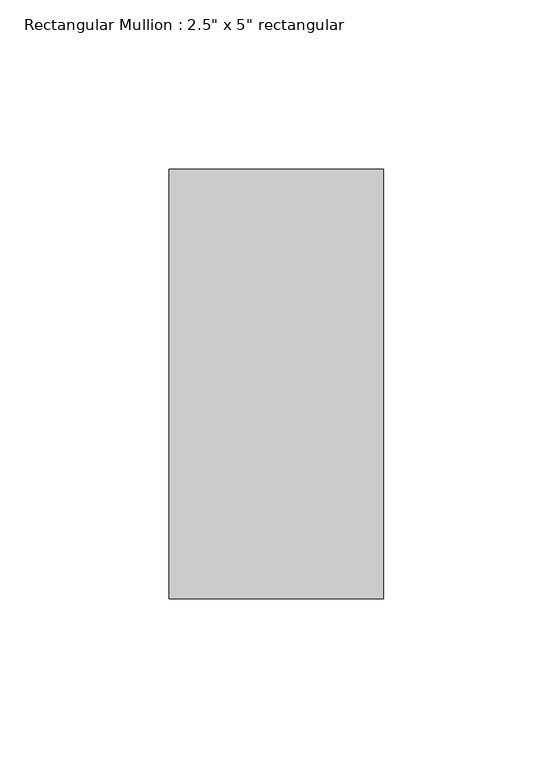
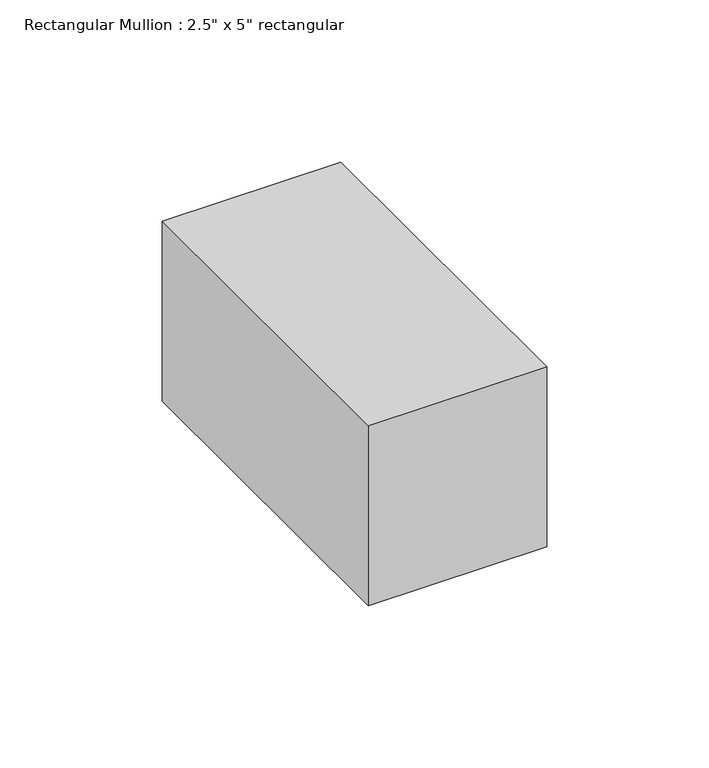
"""IFC4 building model written with IfcOpenShell, lengths in millimetres: member geometry."""

from ifc_helpers import new_model, si_unit, frame, origin, place, context, project, spatial, polyline, outline, extrude, source, transform, mapped, element, save


def member_4a5c7385(model_context):
    return source(origin(), model_context, "Body", "SweptSolid", [
        extrude(outline(polyline([(0.0, 63.5), (0.0, -63.5), (-63.5, -63.5), (-63.5, 63.5), (0.0, 63.5)])), frame((0.0, 0.0, -67.7333333), z_axis=(0.0, 0.0, 1.0), x_axis=(1.0, 0.0, 0.0)), (0.0, 0.0, 1.0), 67.7333333),
    ])


if __name__ == "__main__":
    model = new_model("IFC4")
    model_context = context("Model", 3, world=origin())
    ifc_project = project(units=[si_unit("LENGTHUNIT", "METRE", prefix="MILLI")], contexts=[model_context])
    site = spatial("IfcSite", under=ifc_project)
    building = spatial("IfcBuilding", under=site)
    placement = place(None, origin())
    member_shape = member_4a5c7385(model_context)
    element("IfcMember", 1, ObjectType="Rectangular Mullion : 2.5\" x 5\" rectangular", at=placement, inside=building, context=model_context, shape_type="MappedRepresentation", body=[
        mapped(member_shape, transform((0.0, 0.0, 0.0), x_axis=(1.0, 0.0, 0.0), y_axis=(0.0, 1.0, 0.0), z_axis=(0.0, 0.0, 1.0))),
    ])
    save(model, "model.ifc")

# Revit data of these elements
# Type "Rectangular Mullion : 2.5\" x 5\" rectangular"
#   built-in parameter 1007304 = 0.416667 (stored number, unit not read)
#   built-in parameter 1007301 = 0.104167 (stored number, unit not read)
#   built-in parameter 1007300 = 0.104167 (stored number, unit not read)
# Element 1 (IfcMember, "Rectangular Mullion : 2.5\" x 5\" rectangular")
#   Materials on its faces: "Aluminum"
# Materials
#   "Aluminum": class "Metal", colour RGB 247 247 247, transparency 0, Description = "Aluminum 6061", Cost = 0
